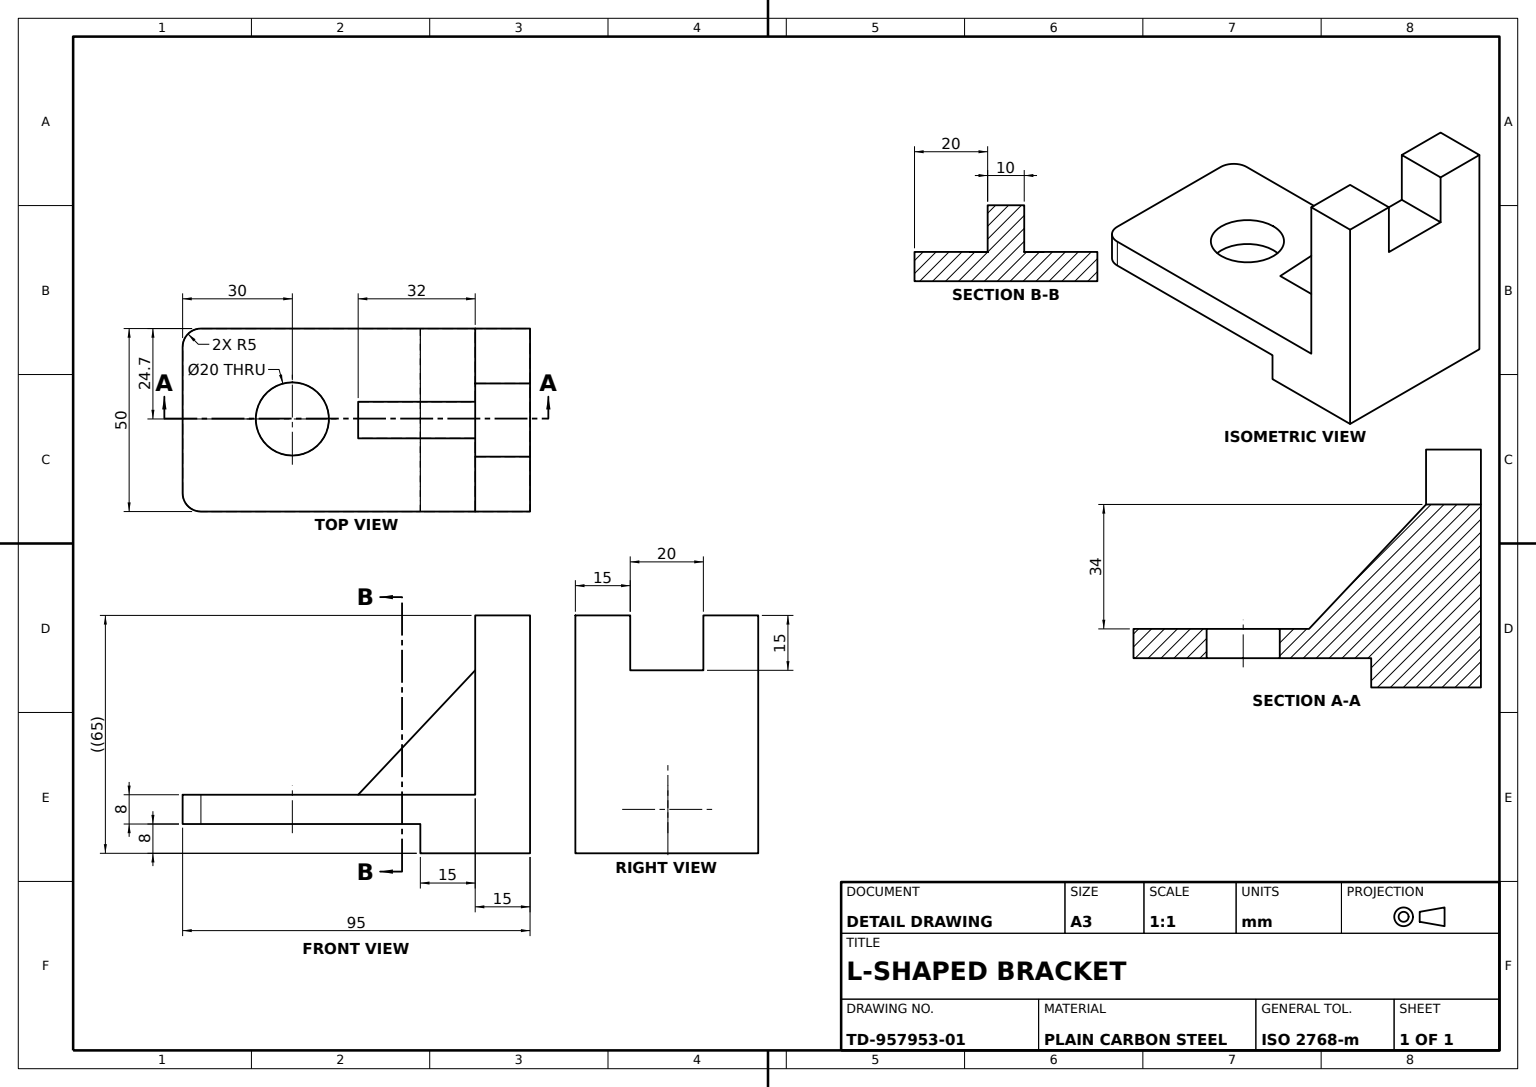
SolidWorks part; units mm, degrees
material "Plain Carbon Steel"
ref_plane "Front Plane" through (0, 0, 0) normal (0, 0, 1) x (1, 0, 0)
ref_plane "Top Plane" through (0, 0, 0) normal (0, 1, 0) x (1, 0, 0)
ref_plane "Right Plane" through (0, 0, 0) normal (1, 0, 0) x (0, 0, -1)
sketch "Bracket L-Profile Sketch" plane through (0, 0, 0) normal (0, 0, 1) x (1, 0, 0)
  line L0 (0, 65) -> (0, 0)
  line L1 (0, 0) -> (-30, 0)
  line L2 (-30, 0) -> (-30, 8)
  line L3 (-30, 8) -> (-95, 8)
  line L4 (-95, 8) -> (-95, 16)
  line L5 (-95, 16) -> (-15, 16)
  line L6 (-15, 16) -> (-15, 65)
  line L7 (-15, 65) -> (0, 65)
  dimension "D1" = 30
  dimension "D2" = 65
  dimension "D3" = 8
  dimension "D4" = 8
  dimension "D5" = 65
  dimension "D6" = 15
extrude "Bracket Body" add sketch "Bracket L-Profile Sketch" along normal blind 50
sketch "Through Hole Sketch" plane through (0, 16, 0) normal (0, 1, 0) x (1, 0, 0)
  line L0 (-95, -50) -> (-95, 0) construction
  line L1 (-15, 0) -> (-95, 0) construction
  circle A0 centre (-65, -24.7006) radius 10
  dimension "D1" = 20
  dimension "D2" = 30
  dimension "D3" = 24.7006
extrude "Through Hole" cut sketch "Through Hole Sketch" against normal blind 50
sketch "Upright Notch Sketch" plane through (0, 65, 0) normal (0, 1, 0) x (1, 0, 0)
  line L1 (0, -25) -> (0, -35)
  line L2 (0, -50) -> (0, 0) construction
  line L3 (0, -35) -> (-15, -35)
  line L4 (-15, -50) -> (-15, 0) construction
  line L5 (-15, -35) -> (-15, -15)
  line L6 (-15, -15) -> (0, -15)
  line L7 (0, -15) -> (0, -25)
  dimension "D1" = 20
  dimension "D2" = 10
extrude "Upright Notch 20x10" cut sketch "Upright Notch Sketch" against normal blind 15
fillet "Corner Fillet R5" radius 5 2 edges at (-95, 12, 0) (-95, 12, 50)
ref_plane "Side Tab Plane" through (0, 0, 25) normal (0, 0, -1) x (-1, 0, 0)
sketch "Side Tab Sketch" plane through (0, 0, 25) normal (0, 0, -1) x (-1, 0, 0)
  line L0 (15, 16) -> (47, 16)
  line L1 (15, 16) -> (90, 16) construction
  line L2 (15, 16) -> (15, 50)
  line L3 (15, 65) -> (15, 16) construction
  line L4 (15, 50) -> (47, 16)
  dimension "D1" = 32
  dimension "D2" = 34
extrude "Side Tab" add sketch "Side Tab Sketch" along normal mid plane 10
